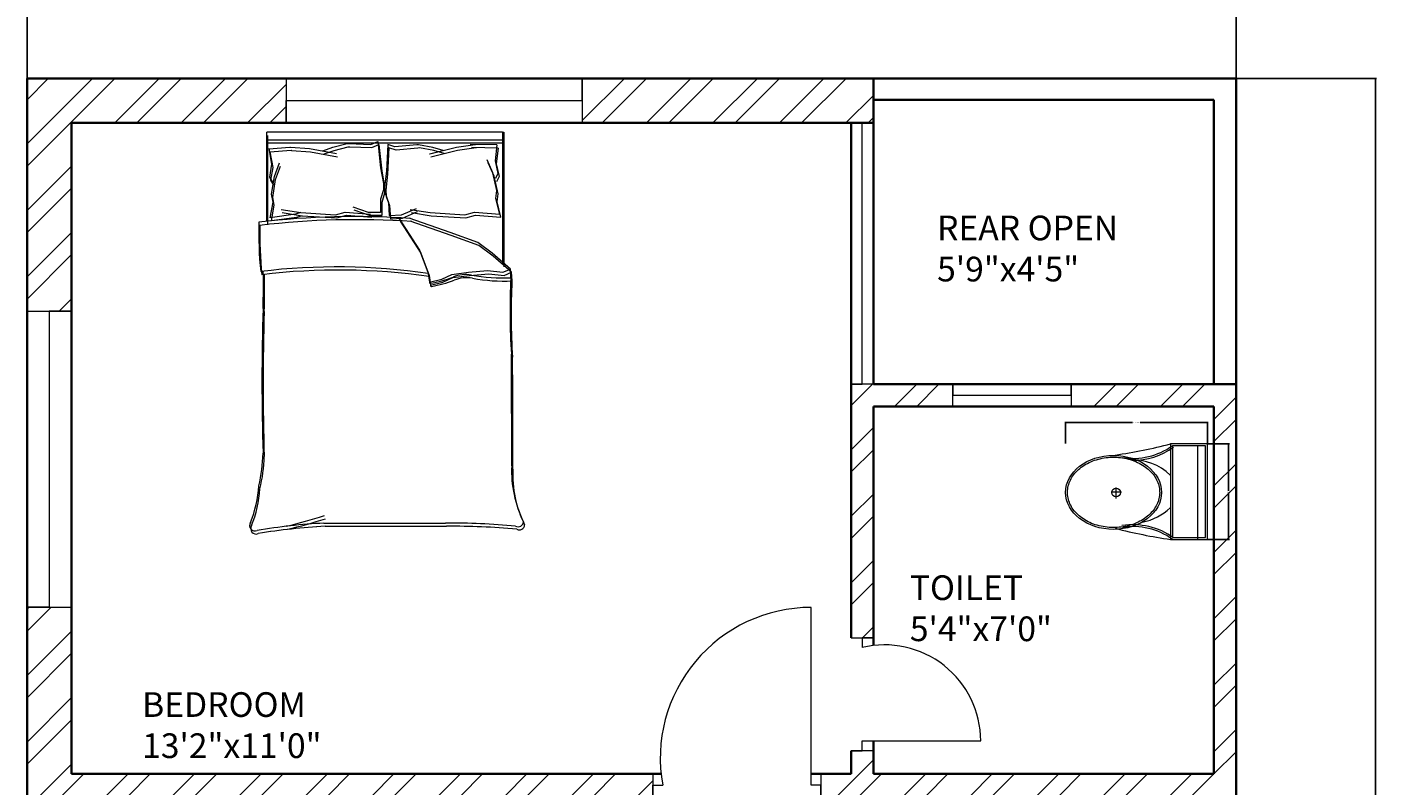
# Model space of a CAD drawing. Units: inches. Extents: x 1850 to 3445, y 1558 to 2756.
# Tile 7 of 13: x 2351 to 2625, y 2073 to 2227. Entities that reach past the tile are written whole.
import ezdxf

# ---------------------------------------------------------------- set-up
doc = ezdxf.new("R2010")
doc.units = ezdxf.units.IN
for name, color, linetype, lineweight in [('A-ANNO-DIMS', 2, 'Continuous', 18), ('A-AREA-IDEN', 7, 'Continuous', 18), ('A-DOOR', 3, 'Continuous', 18), ('A-FLOR-FIXT', 9, 'Continuous', 18), ('A-FURN', 8, 'Continuous', 13), ('A-GLAZ', 4, 'Continuous', 18), ('A-WALL', 7, 'Continuous', 35), ('A-WALL-PATT', 252, 'Continuous', 13)]:
    doc.layers.add(name, color=color, linetype=linetype, lineweight=lineweight)
doc.styles.get("Standard").update_dxf_attribs({"font": 'arial.ttf'})
doc.dimstyles.get("Standard").update_dxf_attribs({"dimtxt": 0.18, "dimasz": 0.18, "dimexe": 0.18, "dimexo": 0.0625, "dimgap": 0.09, "dimtad": 0, "dimtih": 1, "dimtoh": 1, "dimdec": 4, "dimzin": 0, "dimdsep": 46, "dimtxsty": 'Standard', "dimcen": 0.09, "dimadec": 0, "dimazin": 0, "dimtfac": 1, "dimtdec": 4, "dimtofl": 0, "dimtmove": 0, "dimatfit": 3, "dimfxl": 1, "dimtolj": 1, "dimtzin": 0, "dimarcsym": 0})

# ---------------------------------------------------------------- blocks, each defined once
blk = doc.blocks.new('A$C31115884')
for p, q in [((257.5, 466.4), (257.5, 523.2)), ((283.1, 497.7), (223.4, 497.7)), ((0, 200), (0, 0)), ((520, 200), (0, 200)), ((10, 190), (10, 10)), ((510, 190), (10, 190)), ((510, 10), (510, 190)), ((520, 0), (520, 200)), ((510, 54.5), (0, 54.5)), ((10, 10), (510, 10)), ((0, 0), (520, 0))]:
    blk.add_line(p, q)
blk.add_circle((255.6, 496.4), 23.6)
for centre, radius, start, end in [((2777.7, -204.6), 2807, 165.4549, 171.71327), ((-294.5, 403.3), 364.7, 324.20913, 9.34987), ((-294.5, 403.3), 374.7, 324.20913, 9.34987), ((805.8, 403.3), 364.7, 170.65013, 215.79087), ((3237, 905), 2807, 188.28673, 194.5451), ((139.5, 406.2), 293.5, 315.84364, 2.65635), ((805.8, 403.3), 374.7, 179.20365, 215.79087), ((383.6, 406.2), 293.5, 190.27735, 224.15636)]:
    blk.add_arc(centre, radius, start, end)
blk.add_ellipse((256.2, 509.9), major_axis=(0, -260.7), ratio=0.772727)
blk.add_open_spline([(256.2, 259.2), (263.1, 259.2), (270, 259.7), (287.8, 262.3), (298.7, 265.1), (319.9, 273.1), (330.2, 278.4), (350.1, 291.1), (359.7, 298.7), (377.7, 315.9), (386.2, 325.5), (401.7, 346.6), (408.8, 358.1), (421.3, 382.5), (426.8, 395.5), (435.9, 422.4), (439.5, 436.4), (444.8, 465.1), (446.5, 479.7), (447.9, 509.2), (447.6, 524), (445, 553.3), (442.7, 567.8), (436.3, 596), (432.1, 609.7), (421.9, 636), (416, 648.6), (402.5, 672.1), (395, 683), (378.6, 703), (369.8, 712.1), (351.1, 728), (341.3, 734.8), (320.9, 746.2), (310.4, 750.7), (288.9, 757.3), (278, 759.4), (256, 761), (245, 760.6), (223.1, 757.2), (212.3, 754.3), (191.1, 746.1), (180.8, 740.7), (160.9, 727.8), (151.4, 720.1), (133.5, 702.7), (125.1, 693), (109.6, 671.7), (102.6, 660.2), (90.2, 635.7), (84.9, 622.7), (76, 595.6), (72.4, 581.6), (67.2, 552.9), (65.6, 538.2), (64.4, 508.8), (64.8, 494), (67.5, 464.7), (69.9, 450.2), (76.6, 422), (80.8, 408.3), (91.1, 382.2), (97.2, 369.7), (110.8, 346.3), (118.4, 335.4), (134.8, 315.6), (143.7, 306.7), (162.4, 290.9), (172.3, 284.2), (192.8, 273), (203.3, 268.6), (224.8, 262.2), (235.8, 260.2), (249.9, 259.3), (253, 259.2), (256.2, 259.2)], degree=3, knots=[0, 0, 0, 0, 0.110105, 0.110105, 0.285049, 0.285049, 0.459994, 0.459994, 0.634938, 0.634938, 0.809882, 0.809882, 0.984827, 0.984827, 1.159771, 1.159771, 1.334715, 1.334715, 1.50966, 1.50966, 1.684604, 1.684604, 1.859549, 1.859549, 2.034493, 2.034493, 2.209437, 2.209437, 2.384382, 2.384382, 2.559326, 2.559326, 2.73427, 2.73427, 2.909215, 2.909215, 3.084159, 3.084159, 3.259103, 3.259103, 3.434048, 3.434048, 3.608992, 3.608992, 3.783936, 3.783936, 3.958881, 3.958881, 4.133825, 4.133825, 4.30877, 4.30877, 4.483714, 4.483714, 4.658658, 4.658658, 4.833603, 4.833603, 5.008547, 5.008547, 5.183491, 5.183491, 5.358436, 5.358436, 5.53338, 5.53338, 5.708324, 5.708324, 5.883269, 5.883269, 6.058213, 6.058213, 6.233158, 6.233158, 6.283185, 6.283185, 6.283185, 6.283185])
blk = doc.blocks.new('BED-PLAN')
for p, q in [((3.47, 63.33), (3.47, 81.44)), ((3.47, 79.91), (51.27, 79.91)), ((3.48, 63.33), (3.48, 81.44)), ((51.27, 81.44), (3.48, 81.44)), ((3.48, 79.91), (51.27, 79.91)), ((3.7, 62.69), (3.7, 80.8)), ((3.7, 62.69), (3.7, 80.8)), ((24.54, 78.99), (25.98, 79.57)), ((24.54, 78.99), (25.98, 79.57)), ((25.98, 79.57), (26.56, 74.22)), ((25.98, 79.57), (26.56, 74.22)), ((51.27, 81.44), (51.27, 54.83)), ((51.27, 81.44), (51.27, 54.83)), ((51.27, 81.44), (51.49, 81.44)), ((51.49, 81.44), (51.49, 80.8)), ((51.49, 80.8), (51.49, 54.19)), ((51.49, 80.8), (51.49, 54.19)), ((3.7, 79.27), (51.49, 79.27)), ((3.7, 79.27), (51.49, 79.27)), ((3.89, 78.13), (4.47, 74.95)), ((3.89, 78.13), (4.47, 74.95)), ((3.9, 78.11), (8.18, 78.43)), ((3.9, 78.11), (8.18, 78.43)), ((4.12, 77.49), (4.7, 74.31)), ((4.12, 77.49), (4.7, 74.31)), ((4.13, 77.47), (8.41, 77.8)), ((4.13, 77.47), (8.41, 77.8)), ((8.18, 78.43), (8.28, 78.42)), ((8.18, 78.43), (8.28, 78.42)), ((8.28, 78.42), (12.11, 78.13)), ((8.28, 78.42), (12.11, 78.13)), ((8.41, 77.8), (8.51, 77.78)), ((8.41, 77.8), (8.51, 77.78)), ((8.51, 77.78), (12.34, 77.49)), ((8.51, 77.78), (12.34, 77.49)), ((12.11, 78.13), (17.6, 77.11)), ((12.11, 78.13), (17.6, 77.11)), ((12.34, 77.49), (17.83, 76.48)), ((12.34, 77.49), (17.83, 76.48)), ((14.85, 77.69), (16.88, 78.42)), ((14.86, 77.69), (16.88, 78.42)), ((15.08, 77.05), (17.11, 77.78)), ((15.08, 77.05), (17.11, 77.78)), ((16.88, 78.42), (19.77, 79.14)), ((16.88, 78.42), (19.77, 79.14)), ((17.11, 77.78), (20, 78.5)), ((17.11, 77.78), (20, 78.5)), ((19.77, 79.14), (20.09, 79.14)), ((19.77, 79.14), (20.09, 79.14)), ((20, 78.5), (20.32, 78.5)), ((20, 78.5), (20.32, 78.5)), ((20.09, 79.14), (24.54, 78.99)), ((20.09, 79.14), (24.54, 78.99)), ((20.32, 78.5), (24.77, 78.36)), ((20.32, 78.5), (24.77, 78.36)), ((24.77, 78.36), (26.21, 78.93)), ((24.77, 78.36), (26.21, 78.93)), ((26.21, 78.93), (26.79, 73.58)), ((26.21, 78.93), (26.79, 73.58)), ((27.98, 78.95), (27.73, 73.58)), ((27.98, 78.95), (27.73, 73.58)), ((28.21, 78.31), (27.96, 72.94)), ((28.21, 78.31), (27.96, 72.94)), ((29.46, 78.46), (27.98, 78.95)), ((29.46, 78.46), (27.98, 78.95)), ((29.68, 77.83), (28.21, 78.31)), ((29.68, 77.83), (28.21, 78.31)), ((33.88, 78.89), (29.46, 78.46)), ((33.88, 78.89), (29.46, 78.46)), ((34.11, 78.25), (29.68, 77.83)), ((34.11, 78.25), (29.68, 77.83)), ((34.2, 78.91), (33.88, 78.89)), ((34.2, 78.91), (33.88, 78.89)), ((34.43, 78.27), (34.11, 78.25)), ((34.43, 78.27), (34.11, 78.25)), ((37.14, 78.36), (34.2, 78.91)), ((37.14, 78.36), (34.2, 78.91)), ((37.36, 77.73), (34.43, 78.27)), ((37.36, 77.73), (34.43, 78.27)), ((41.91, 78.37), (36.49, 77.02)), ((41.91, 78.37), (36.5, 77.02)), ((42.14, 77.73), (36.72, 76.38)), ((42.14, 77.73), (36.72, 76.38)), ((39.2, 77.77), (37.14, 78.36)), ((39.2, 77.77), (37.14, 78.36)), ((39.43, 77.13), (37.36, 77.73)), ((39.43, 77.13), (37.36, 77.73)), ((45.71, 78.9), (41.91, 78.37)), ((45.71, 78.9), (41.91, 78.37)), ((45.94, 78.26), (42.14, 77.73)), ((45.94, 78.26), (42.14, 77.73)), ((50.11, 78.89), (44.71, 78.98)), ((44.71, 78.98), (45.71, 78.9)), ((50.11, 78.89), (44.71, 78.98)), ((44.71, 78.98), (45.71, 78.9)), ((50.34, 78.25), (44.94, 78.34)), ((44.94, 78.34), (45.94, 78.26)), ((50.34, 78.25), (44.94, 78.34)), ((44.94, 78.34), (45.94, 78.26)), ((50.11, 78.89), (49.73, 75.68)), ((50.11, 78.89), (49.73, 75.68)), ((50.34, 78.25), (49.96, 75.04)), ((50.34, 78.25), (49.96, 75.04)), ((4.47, 74.95), (4.04, 72.34)), ((4.47, 74.95), (4.04, 72.34)), ((4.7, 74.31), (4.27, 71.7)), ((4.7, 74.31), (4.27, 71.7)), ((5.05, 72.49), (6.06, 75.24)), ((5.05, 72.49), (6.06, 75.24)), ((5.28, 71.85), (6.29, 74.6)), ((5.28, 71.85), (6.29, 74.6)), ((26.56, 74.22), (27.14, 71.04)), ((26.56, 74.22), (27.14, 71.04)), ((49.31, 73.19), (48.13, 75.86)), ((49.31, 73.19), (48.13, 75.86)), ((49.54, 72.55), (48.36, 75.23)), ((49.54, 72.55), (48.36, 75.23)), ((49.73, 75.68), (50.33, 73.1)), ((49.73, 75.68), (50.33, 73.1)), ((49.96, 75.04), (50.56, 72.47)), ((49.96, 75.04), (50.56, 72.47)), ((4.04, 72.34), (4.62, 71.33)), ((4.04, 72.34), (4.62, 71.33)), ((4.27, 71.7), (4.85, 70.69)), ((4.27, 71.7), (4.85, 70.69)), ((4.47, 68.87), (5.05, 72.49)), ((4.47, 68.87), (5.05, 72.49)), ((4.7, 68.23), (5.28, 71.85)), ((4.7, 68.23), (5.28, 71.85)), ((26.79, 73.58), (27.37, 70.4)), ((26.79, 73.58), (27.37, 70.4)), ((27.73, 73.58), (27.35, 70.37)), ((27.73, 73.58), (27.35, 70.37)), ((27.96, 72.94), (27.58, 69.73)), ((27.96, 72.94), (27.58, 69.73)), ((50.11, 69.61), (49.31, 73.19)), ((50.11, 69.61), (49.31, 73.19)), ((50.34, 68.98), (49.54, 72.55)), ((50.34, 68.98), (49.54, 72.55)), ((50.33, 73.1), (49.81, 72.06)), ((50.33, 73.1), (49.81, 72.06)), ((50.56, 72.47), (50.04, 71.42)), ((50.56, 72.47), (50.04, 71.42)), ((4.76, 67.28), (4.47, 68.87)), ((4.76, 67.28), (4.47, 68.87)), ((27.14, 69.74), (26.56, 67.86)), ((27.14, 69.74), (26.56, 67.86)), ((27.37, 69.1), (26.79, 67.22)), ((27.37, 69.1), (26.79, 67.22)), ((27.14, 71.04), (27.14, 69.74)), ((27.14, 71.04), (27.14, 69.74)), ((27.35, 70.37), (27.44, 69.07)), ((27.35, 70.37), (27.44, 69.07)), ((27.37, 70.4), (27.37, 69.1)), ((27.37, 70.4), (27.37, 69.1)), ((27.44, 69.07), (28.13, 67.23)), ((27.44, 69.07), (28.13, 67.23)), ((27.58, 69.73), (27.66, 68.43)), ((27.58, 69.73), (27.66, 68.43)), ((27.66, 68.43), (28.36, 66.59)), ((27.66, 68.43), (28.36, 66.59)), ((49.92, 68.01), (50.11, 69.61)), ((49.92, 68.01), (50.11, 69.61)), ((50.15, 67.37), (50.34, 68.98)), ((50.15, 67.37), (50.34, 68.98)), ((4.18, 64.1), (4.76, 67.28)), ((4.18, 64.1), (4.76, 67.28)), ((4.41, 63.46), (4.99, 66.64)), ((4.41, 63.46), (4.99, 66.64)), ((4.99, 66.64), (4.7, 68.23)), ((4.99, 66.64), (4.7, 68.23)), ((6.38, 65.81), (10.41, 65.15)), ((6.38, 65.81), (10.41, 65.15)), ((24.1, 65.18), (20.96, 66.27)), ((24.1, 65.18), (20.96, 66.27)), ((26.56, 67.86), (26.56, 65.18)), ((26.56, 67.86), (26.56, 65.18)), ((26.79, 67.22), (26.79, 64.54)), ((26.79, 67.22), (26.79, 64.54)), ((28.13, 67.23), (28.3, 64.55)), ((28.13, 67.23), (28.3, 64.55)), ((28.36, 66.59), (28.53, 63.91)), ((28.36, 66.59), (28.53, 63.91)), ((30.75, 64.7), (33.82, 65.99)), ((30.75, 64.7), (33.82, 65.99)), ((32.56, 65.81), (36.6, 65.15)), ((32.56, 65.81), (36.6, 65.15)), ((50.7, 64.87), (49.92, 68.01)), ((50.7, 64.87), (49.92, 68.01)), ((50.93, 64.23), (50.15, 67.37)), ((50.93, 64.23), (50.15, 67.37)), ((9.28, 64.83), (4.18, 64.1)), ((9.28, 64.83), (4.18, 64.1)), ((9.51, 64.19), (4.41, 63.46)), ((9.51, 64.19), (4.41, 63.46)), ((6.61, 65.18), (10.64, 64.51)), ((6.61, 65.18), (10.64, 64.51)), ((10.41, 65.15), (9.28, 64.83)), ((10.41, 65.15), (9.28, 64.83)), ((10.64, 64.51), (9.51, 64.19)), ((10.64, 64.51), (9.51, 64.19)), ((10.41, 65.15), (17.42, 64.72)), ((10.41, 65.15), (17.42, 64.72)), ((10.64, 64.51), (17.65, 64.08)), ((10.64, 64.51), (17.65, 64.08)), ((17.42, 64.72), (19.38, 65.27)), ((17.42, 64.72), (19.38, 65.27)), ((17.65, 64.08), (19.61, 64.63)), ((17.65, 64.08), (19.61, 64.63)), ((19.38, 65.27), (24.52, 64.87)), ((19.38, 65.27), (24.52, 64.87)), ((19.61, 64.63), (24.74, 64.23)), ((19.61, 64.63), (24.74, 64.23)), ((24.33, 64.54), (21.19, 65.63)), ((24.33, 64.54), (21.19, 65.63)), ((26.56, 65.18), (24.1, 65.18)), ((26.56, 65.18), (24.1, 65.18)), ((26.79, 64.54), (24.33, 64.54)), ((26.79, 64.54), (24.33, 64.54)), ((28.3, 64.55), (30.75, 64.7)), ((28.3, 64.55), (30.75, 64.7)), ((28.53, 63.91), (30.98, 64.06)), ((28.53, 63.91), (30.98, 64.06)), ((30.26, 64.06), (34.45, 57.57)), ((30.26, 64.06), (34.45, 57.57)), ((30.49, 63.42), (34.68, 56.93)), ((30.49, 63.42), (34.68, 56.93)), ((30.98, 64.06), (34.05, 65.35)), ((30.98, 64.06), (34.05, 65.35)), ((40.64, 61.13), (32.31, 64.06)), ((40.64, 61.13), (32.31, 64.06)), ((40.87, 60.49), (32.53, 63.42)), ((40.87, 60.49), (32.53, 63.42)), ((32.79, 65.18), (36.82, 64.51)), ((32.79, 65.18), (36.82, 64.51)), ((36.6, 65.15), (43.61, 64.72)), ((36.6, 65.15), (43.61, 64.72)), ((36.82, 64.51), (43.83, 64.08)), ((36.82, 64.51), (43.83, 64.08)), ((43.61, 64.72), (45.57, 65.27)), ((43.61, 64.72), (45.57, 65.27)), ((43.83, 64.08), (45.79, 64.63)), ((43.83, 64.08), (45.79, 64.63)), ((45.57, 65.27), (50.7, 64.87)), ((45.57, 65.27), (50.7, 64.87)), ((45.79, 64.63), (50.93, 64.23)), ((45.79, 64.63), (50.93, 64.23)), ((46.22, 59.11), (40.64, 61.13)), ((46.22, 59.11), (40.64, 61.13)), ((46.45, 58.48), (40.87, 60.49)), ((46.45, 58.48), (40.87, 60.49)), ((34.45, 57.57), (36.15, 53.08)), ((34.45, 57.57), (36.15, 53.08)), ((49.16, 56.95), (46.22, 59.11)), ((49.16, 56.95), (46.22, 59.11)), ((49.39, 56.31), (46.45, 58.48)), ((49.39, 56.31), (46.45, 58.48)), ((34.68, 56.93), (36.38, 52.44)), ((34.68, 56.93), (36.38, 52.44)), ((52.87, 53.7), (49.16, 56.95)), ((52.87, 53.7), (49.16, 56.95)), ((53.1, 53.06), (49.39, 56.31)), ((53.1, 53.06), (49.39, 56.31)), ((36.15, 53.08), (36.46, 51.07)), ((36.15, 53.08), (36.46, 51.07)), ((36.38, 52.44), (36.69, 50.43)), ((36.38, 52.44), (36.69, 50.43)), ((38.94, 51.69), (40.95, 52.61)), ((38.94, 51.69), (40.95, 52.61)), ((40.95, 52.61), (44.36, 53.08)), ((40.95, 52.61), (44.36, 53.08)), ((41.18, 51.97), (44.59, 52.44)), ((41.18, 51.97), (44.59, 52.44)), ((44.36, 53.08), (48.23, 53.39)), ((44.36, 53.08), (48.23, 53.39)), ((44.59, 52.44), (48.46, 52.75)), ((44.59, 52.44), (48.46, 52.75)), ((48.23, 53.39), (51.33, 53.08)), ((48.23, 53.39), (51.33, 53.08)), ((48.46, 52.75), (51.56, 52.44)), ((48.46, 52.75), (51.56, 52.44)), ((51.33, 53.08), (52.87, 53.7)), ((51.33, 53.08), (52.87, 53.7)), ((51.56, 52.44), (53.1, 53.06)), ((51.56, 52.44), (53.1, 53.06)), ((52.95, 51.95), (52.87, 53.7, 3.87)), ((52.95, 51.95), (52.87, 53.7, 3.87)), ((53.18, 51.31), (53.1, 53.06, 3.87)), ((53.18, 51.31), (53.1, 53.06, 3.87)), ((36.46, 51.07), (38.94, 51.69)), ((36.46, 51.07), (38.94, 51.69)), ((36.69, 50.43), (39.17, 51.05)), ((36.69, 50.43), (39.17, 51.05)), ((39.17, 51.05), (41.18, 51.97)), ((39.17, 51.05), (41.18, 51.97)), ((15.06, 2.2), (39.68, 2.2)), ((15.06, 2.2), (39.68, 2.2)), ((15.29, 1.56), (39.91, 1.56)), ((15.29, 1.56), (39.91, 1.56))]:
    blk.add_line(p, q)
for centre, radius, start, end in [((85.16, 61.35), 83.31, 178.7218, 185.604), ((85.16, 61.35), 83.31, 178.7218, 185.604), ((21.36, -100.61), 164.97, 86.0865, 96.7821), ((21.36, -100.61), 164.97, 86.0865, 96.7821), ((21.59, -101.25), 164.97, 86.0865, 96.7821), ((21.59, -101.25), 164.97, 86.0865, 96.7821), ((85.39, 60.71), 83.31, 178.7218, 185.604), ((85.39, 60.71), 83.31, 178.7218, 185.604), ((17.76, -74.87), 129.02, 81.7845, 96.9006), ((17.76, -74.87), 129.02, 81.7845, 96.9006), ((17.98, -75.51), 129.02, 81.7845, 96.9006), ((17.98, -75.51), 129.02, 81.7845, 96.9006), ((-167.31, 50.27), 170.11, 358.4762, 1.0082), ((-167.31, 50.27), 170.11, 358.4762, 1.0082), ((-167.08, 49.63), 170.11, 358.4762, 1.0082), ((-167.08, 49.63), 170.11, 358.4762, 1.0082), ((31.15, 79.96), 29.65, 280.6617, 289.8806), ((31.15, 79.96), 29.65, 280.6617, 289.8806), ((43.74, 46.38), 6.22, 78.6608, 113.7384), ((43.74, 46.38), 6.22, 78.6608, 113.7384), ((51.33, 88.1), 36.18, 259.8763, 272.5657), ((51.33, 88.1), 36.18, 259.8763, 272.5657), ((36.64, 51), 0.185, 160.2464, 271.1377), ((36.64, 51), 0.185, 160.2464, 271.1377), ((36.86, 50.36), 0.185, 160.2464, 271.1377), ((36.86, 50.36), 0.185, 160.2464, 271.1377), ((31.38, 79.32), 29.65, 280.6617, 289.8806), ((31.38, 79.32), 29.65, 280.6617, 289.8806), ((43.97, 45.74), 6.22, 78.6608, 113.7384), ((43.97, 45.74), 6.22, 78.6608, 113.7384), ((51.56, 87.46), 36.18, 259.8763, 272.5657), ((51.56, 87.46), 36.18, 259.8763, 272.5657), ((182.27, 45.13), 129.5, 176.9791, 183.8365), ((182.27, 45.13), 129.5, 176.9791, 183.8365), ((182.49, 44.49), 129.5, 176.9791, 183.8365), ((182.49, 44.49), 129.5, 176.9791, 183.8365), ((484.82, 30.83), 482.31, 178.2277, 181.7185), ((484.82, 30.83), 482.31, 178.2277, 181.7185), ((485.05, 30.19), 482.31, 178.2277, 181.7185), ((485.05, 30.19), 482.31, 178.2277, 181.7185), ((-4508.74, 13.62), 4561.86, 0.00217, 0.28689), ((-4508.74, 13.62), 4561.86, 0.00217, 0.28689), ((-4508.51, 12.98), 4561.86, 0.00217, 0.28689), ((-4508.52, 12.98), 4561.86, 0.00217, 0.28689), ((-26.9, 16.93), 29.63, 346.0648, 358.9113), ((-26.9, 16.93), 29.63, 346.0648, 358.9113), ((-26.67, 16.29), 29.63, 346.0648, 358.9113), ((-26.67, 16.29), 29.63, 346.0648, 358.9113), ((76.16, 12.78), 23.07, 177.4714, 206.4681), ((76.16, 12.78), 23.07, 177.4714, 206.4681), ((76.39, 12.14), 23.07, 177.4714, 206.4681), ((76.39, 12.14), 23.07, 177.4714, 206.4681), ((-21.66, 11.17), 23.56, 337.9751, 356.652), ((-21.66, 11.17), 23.56, 337.9751, 356.652), ((-21.43, 10.53), 23.56, 337.9751, 356.652), ((-21.43, 10.53), 23.56, 337.9751, 356.652), ((-17.22, 105.16), 106.46, 283.3832, 287.7053), ((-17.22, 105.16), 106.46, 283.3832, 287.7053), ((-16.99, 104.52), 106.46, 283.3832, 287.7053), ((-16.99, 104.52), 106.46, 283.3832, 287.7053), ((1.09, 1.73), 1.09, 146.1736, 293.4781), ((1.09, 1.73), 1.09, 146.1736, 293.4781), ((1.32, 1.09), 1.09, 146.1736, 293.4781), ((1.32, 1.09), 1.09, 146.1736, 293.4781), ((21.43, -119.39), 121.76, 92.9958, 99.4091), ((21.43, -119.39), 121.76, 92.9958, 99.4091), ((21.66, -120.03), 121.76, 92.9958, 99.4091), ((21.65, -120.03), 121.76, 92.9958, 99.4091), ((41.15, -130.83), 133.04, 84.4998, 90.6351), ((41.15, -130.83), 133.04, 84.4998, 90.6351), ((41.38, -131.47), 133.04, 84.4998, 90.6351), ((41.38, -131.47), 133.04, 84.4998, 90.6351), ((54.41, 2.57), 1.1, 242.6588, 356.02), ((54.41, 2.57), 1.1, 242.6588, 356.02), ((54.64, 1.93), 1.1, 242.6588, 356.02), ((54.64, 1.93), 1.1, 242.6588, 356.02)]:
    blk.add_arc(centre, radius, start, end)
blk = doc.blocks.new('WIN-60-W9')
for p, q in [((0, 9), (0, 0)), ((60, 4.5), (60, 9)), ((60, 9), (60, 0)), ((0, 0), (0, 4.5)), ((0, 4.5), (60, 4.5))]:
    blk.add_line(p, q)
blk = doc.blocks.new('WIN-24-W4_5')
for p, q in [((0, 0), (0, 4.5)), ((0, 4.5), (0, 2.25)), ((24, 2.25), (24, 4.5)), ((24, 4.5), (24, 0)), ((0, 2.25), (24, 2.25))]:
    blk.add_line(p, q)
blk = doc.blocks.new('DOOR-BATH-REAR-UPPER')
for p, q in [((0, 22.93), (4.5, 22.93)), ((4.5, 22.93), (2.25, 22.93)), ((2.25, 22.93), (2.25, 20.93)), ((2.25, 0), (2.25, 2)), ((2.25, 2), (26.25, 2)), ((4.5, 0), (0, 0)), ((0, 0), (2.25, 0))]:
    blk.add_line(p, q)
blk.add_arc((6.78, 2), 19.47, 0, 103.4712)
blk = doc.blocks.new('DOOR-BED-UPPER')
for p, q in [((32.07, 2.25), (32.07, 38.25)), ((0, 4.5), (0, 0)), ((34.07, 4.5), (34.07, 0)), ((0, 0), (0, 2.25)), ((0, 2.25), (2, 2.25)), ((34.07, 2.25), (32.07, 2.25)), ((34.07, 0), (34.07, 2.25))]:
    blk.add_line(p, q)
blk.add_arc((32.07, 7.69), 30.56, 90, 190.2532)
blk = doc.blocks.new('*D48')
at = {"layer": 'A-ANNO-DIMS', "color": 0, "lineweight": -2, "transparency": 16777216}
for p, q in [((2561.52, 2142.15), (2561.52, 2146.58)), ((2561.7, 2146.4), (2575.1, 2146.4)), ((2590.06, 2146.4), (2576.65, 2146.4)), ((2590.24, 2142.15), (2590.24, 2146.58))]:
    blk.add_line(p, q, dxfattribs=at)
at = {"layer": 'A-ANNO-DIMS', "color": 0, "transparency": 16777216}
for points in [[(2561.7, 2146.43), (2561.7, 2146.37), (2561.52, 2146.4)], [(2590.06, 2146.43), (2590.06, 2146.37), (2590.24, 2146.4)]]:
    blk.add_solid(points, dxfattribs=at)
at = {"layer": 'Defpoints', "color": 0, "transparency": 16777216}
for p in [(2561.52, 2146.4), (2561.52, 2142.09), (2590.24, 2142.09)]:
    blk.add_point(p, dxfattribs=at)
at = {"layer": 'A-ANNO-DIMS', "color": 0, "transparency": 16777216, "insert": (2575.88, 2146.4), "char_height": 0.18, "attachment_point": 5}
blk.add_mtext('\\A1;WC 29 TYP.', dxfattribs=at)
blk = doc.blocks.new('*D49')
at = {"layer": 'A-ANNO-DIMS', "color": 0, "lineweight": -2, "transparency": 16777216}
for p, q in [((2590.3, 2142.09), (2594.73, 2142.09)), ((2594.55, 2141.91), (2594.55, 2132.58)), ((2594.55, 2122.89), (2594.55, 2132.22)), ((2590.3, 2122.71), (2594.73, 2122.71))]:
    blk.add_line(p, q, dxfattribs=at)
at = {"layer": 'A-ANNO-DIMS', "color": 0, "transparency": 16777216}
for points in [[(2594.52, 2141.91), (2594.58, 2141.91), (2594.55, 2142.09)], [(2594.52, 2122.89), (2594.58, 2122.89), (2594.55, 2122.71)]]:
    blk.add_solid(points, dxfattribs=at)
at = {"layer": 'Defpoints', "color": 0, "transparency": 16777216}
for p in [(2590.24, 2142.09), (2594.55, 2142.09), (2590.24, 2122.71)]:
    blk.add_point(p, dxfattribs=at)
at = {"layer": 'A-ANNO-DIMS', "color": 0, "transparency": 16777216, "insert": (2594.55, 2132.4), "char_height": 0.18, "attachment_point": 5}
blk.add_mtext('\\A1;19 TYP.', dxfattribs=at)
blk = doc.blocks.new('*D82')
at = {"layer": 'A-ANNO-DIMS', "color": 0, "lineweight": -2, "transparency": 16777216}
for p, q in [((2351.06, 2216.25), (2351.06, 2244.61)), ((2351.24, 2244.43), (2473.26, 2244.43)), ((2595.88, 2244.43), (2473.85, 2244.43)), ((2596.06, 2216.25), (2596.06, 2244.61))]:
    blk.add_line(p, q, dxfattribs=at)
at = {"layer": 'A-ANNO-DIMS', "color": 0, "transparency": 16777216}
for points in [[(2351.24, 2244.46), (2351.24, 2244.4), (2351.06, 2244.43)], [(2595.88, 2244.46), (2595.88, 2244.4), (2596.06, 2244.43)]]:
    blk.add_solid(points, dxfattribs=at)
at = {"layer": 'Defpoints', "color": 0, "transparency": 16777216}
for p in [(2596.06, 2244.43), (2351.06, 2216.18), (2596.06, 2216.18)]:
    blk.add_point(p, dxfattribs=at)
at = {"layer": 'A-ANNO-DIMS', "color": 0, "transparency": 16777216, "insert": (2473.56, 2244.43), "char_height": 0.18, "attachment_point": 5}
blk.add_mtext('\\A1;245', dxfattribs=at)
blk = doc.blocks.new('*D83')
at = {"layer": 'A-ANNO-DIMS', "color": 0, "lineweight": -2, "transparency": 16777216}
for p, q in [((2596.12, 2216.18), (2624.49, 2216.18)), ((2624.31, 2216), (2624.31, 1977.12)), ((2624.31, 1737.86), (2624.31, 1976.75)), ((2596.12, 1737.68), (2624.49, 1737.68))]:
    blk.add_line(p, q, dxfattribs=at)
at = {"layer": 'A-ANNO-DIMS', "color": 0, "transparency": 16777216}
for points in [[(2624.28, 2216), (2624.34, 2216), (2624.31, 2216.18)], [(2624.28, 1737.86), (2624.34, 1737.86), (2624.31, 1737.68)]]:
    blk.add_solid(points, dxfattribs=at)
at = {"layer": 'Defpoints', "color": 0, "transparency": 16777216}
for p in [(2596.06, 2216.18), (2624.31, 2216.18), (2596.06, 1737.68)]:
    blk.add_point(p, dxfattribs=at)
at = {"layer": 'A-ANNO-DIMS', "color": 0, "transparency": 16777216, "insert": (2624.31, 1976.93), "char_height": 0.18, "attachment_point": 5}
blk.add_mtext('\\A1;478.5', dxfattribs=at)

msp = doc.modelspace()

# ---------------------------------------------------------------- hatches: boundary and pattern name
at = {"layer": 'A-WALL-PATT'}
h = msp.add_hatch(dxfattribs=at)
h.set_pattern_fill('ANSI32', color=256)
h.paths.add_polyline_path([(2403.5576, 2211.6843), (2403.5576, 2216.1843), (2351.0556, 2216.1843), (2351.0556, 2169.0079), (2360.0556, 2169.0079), (2360.0556, 2207.1843), (2403.5576, 2207.1843)])
h.paths.add_polyline_path([(2522.5556, 2216.1843), (2463.5576, 2216.1843), (2463.5576, 2207.1843), (2522.5556, 2207.1843)])
h.paths.add_polyline_path([(2596.0556, 2154.1843), (2562.6647, 2154.1843), (2562.6647, 2149.6843), (2591.5556, 2149.6843), (2591.5556, 2075.1843), (2522.5556, 2075.1843), (2522.5556, 2079.8699), (2518.0556, 2079.8699), (2518.0556, 2075.1843), (2511.9412, 2075.1843), (2511.9412, 2070.6843), (2591.5556, 2070.6843), (2591.5556, 2036.4962), (2596.0556, 2036.4962)])
h.paths.add_polyline_path([(2538.6647, 2154.1843), (2522.5556, 2154.1843), (2518.0556, 2154.1843), (2518.0556, 2102.7998), (2522.5556, 2102.7998), (2522.5556, 2149.6843), (2538.6647, 2149.6843)], flags=17)
h.paths.add_polyline_path([(2477.8689, 2072.9343), (2477.8689, 2075.1843), (2360.0556, 2075.1843), (2360.0556, 2109.0079), (2355.5556, 2109.0079), (2351.0556, 2109.0079), (2351.0556, 2043.8694), (2355.5556, 2043.8694), (2360.0556, 2043.8694), (2360.0556, 2070.6843), (2450.0556, 2070.6843), (2450.0556, 2045.0271), (2454.5556, 2045.0271), (2454.5556, 2070.6843), (2477.8689, 2070.6843)])
h.paths.add_polyline_path([(2360.0556, 2007.8694), (2351.0556, 2007.8694), (2351.0556, 1958.9131), (2355.5556, 1958.9131), (2360.0556, 1958.9131), (2360.0556, 1970.1843), (2450.0556, 1970.1843), (2450.0556, 1913.1843), (2443.7332, 1913.1843), (2443.7332, 1908.6843), (2454.5556, 1908.6843), (2454.5556, 1999.4184), (2450.0556, 1999.4184), (2450.0556, 1974.6843), (2360.0556, 1974.6843)])
h.paths.add_polyline_path([(2360.0556, 1908.6843), (2422.4247, 1908.6843), (2422.4247, 1910.9343), (2422.4247, 1913.1843), (2360.0556, 1913.1843), (2360.0556, 1934.9131), (2351.0556, 1934.9131), (2351.0556, 1778.1843), (2426.033, 1778.1843), (2426.033, 1780.4343), (2426.033, 1782.6843), (2360.0556, 1782.6843)])
h.paths.add_polyline_path([(2515.0556, 1782.6843), (2486.033, 1782.6843), (2486.033, 1778.1843), (2515.0556, 1778.1843)])

# ---------------------------------------------------------------- linework, layer by layer
at = {"layer": 'A-GLAZ'}
for p, q in [((2520.3056, 2154.1843), (2520.3056, 2207.1843)), ((2522.5556, 2154.1843), (2518.0556, 2154.1843)), ((2518.0556, 2154.1843), (2520.3056, 2154.1843))]:
    msp.add_line(p, q, dxfattribs=at)
at = {"layer": 'A-WALL'}
for p, q in [((2351.0556, 2216.1843), (2596.0556, 2216.1843)), ((2351.0556, 2216.1843), (2351.0556, 1737.6843)), ((2522.5556, 2216.1843), (2522.5556, 2154.1843)), ((2596.0556, 2216.1843), (2596.0556, 1737.6843)), ((2522.5556, 2211.8264), (2591.5556, 2211.8264)), ((2591.5556, 2211.8264), (2591.5556, 2207.1843)), ((2360.0556, 2207.1843), (2522.5556, 2207.1843)), ((2360.0556, 2207.1843), (2360.0556, 2075.1843)), ((2518.0556, 2207.1843), (2518.0556, 2102.7998)), ((2591.5556, 2207.1843), (2591.5556, 2154.1843)), ((2522.5556, 2154.1843), (2596.0556, 2154.1843)), ((2522.5556, 2149.6843), (2522.5556, 2101.2008)), ((2522.5556, 2149.6843), (2591.5556, 2149.6843)), ((2591.5556, 2149.6843), (2591.5556, 2075.1843)), ((2522.5556, 2081.8699), (2522.5556, 2075.1843)), ((2518.0556, 2079.8699), (2518.0556, 2075.1843)), ((2360.0556, 2075.1843), (2479.5478, 2075.1843)), ((2509.9412, 2075.1843), (2518.0556, 2075.1843)), ((2522.5556, 2075.1843), (2591.5556, 2075.1843))]:
    msp.add_line(p, q, dxfattribs=at)

# ---------------------------------------------------------------- block references
at = {"layer": 'A-DOOR'}
for name, p in [('DOOR-BED-UPPER', (2477.869, 2070.684)), ('DOOR-BATH-REAR-UPPER', (2518.056, 2079.87))]:
    msp.add_blockref(name, p, dxfattribs=at)
at = {"layer": 'A-FLOR-FIXT', "xscale": 0.0372717239612423, "yscale": 0.0372717239612423, "zscale": 0.0372717239612423, "rotation": 89.99999999999999}
msp.add_blockref('A$C31115884', (2590.237, 2122.708), dxfattribs=at)
at = {"layer": 'A-FURN'}
msp.add_blockref('BED-PLAN', (2396.1595, 2123.8152), dxfattribs=at)
at = {"layer": 'A-GLAZ'}
for name, p in [('WIN-60-W9', (2403.5575, 2207.184)), ('WIN-24-W4_5', (2538.665, 2149.684))]:
    msp.add_blockref(name, p, dxfattribs=at)
at = {"layer": 'A-GLAZ', "extrusion": (0, 0, -1), "zscale": -1, "rotation": 270}
msp.add_blockref('WIN-60-W9', (-2360.0559, 2169.008), dxfattribs=at)

# ---------------------------------------------------------------- texts
at = {"layer": 'A-AREA-IDEN', "char_height": 5, "attachment_point": 1}
for s, width, insert in [('REAR OPEN\\P5\'9"x4\'5"', 101.614587, (2535.4723, 2188.358)), ('TOILET\\P5\'4"x7\'0"', 115.801334, (2529.9458, 2115.4354)), ('BEDROOM\\P13\'2"x11\'0"', 157.927169, (2374.3784, 2091.7435))]:
    msp.add_mtext_dynamic_manual_height_columns(s, width=width, gutter_width=12.5, heights=[0], dxfattribs=dict(at, insert=insert))

# ---------------------------------------------------------------- dimensions: what is measured, and where the dimension line sits
at = {"layer": 'A-ANNO-DIMS'}
dim = msp.add_linear_dim(base=(2596.0556, 2244.4343), p1=(2351.0556, 2216.1843), p2=(2596.0556, 2216.1843), dimstyle='Standard', override={"dimdec": 0, "dimlfac": 1, "dimrnd": 0, "dimzin": 0, "dimdsep": 46, "dimlunit": 2}, dxfattribs=at)
dim.commit()
dim.dimension.update_dxf_attribs({"geometry": '*D82', "text_midpoint": (2473.5556, 2244.4343)})
dim = msp.add_linear_dim(base=(2624.3056, 2216.1843), p1=(2596.0556, 1737.6843), p2=(2596.0556, 2216.1843), angle=90, dimstyle='Standard', override={"dimdec": 1, "dimlfac": 1, "dimrnd": 0, "dimzin": 0, "dimdsep": 46, "dimlunit": 2}, dxfattribs=at)
dim.commit()
dim.dimension.update_dxf_attribs({"geometry": '*D83', "text_midpoint": (2624.3056, 1976.9343)})
for base, p1, p2, angle, text, picture, middle in [((2561.5165, 2146.3974), (2590.237, 2142.0893), (2561.5165, 2142.0893), 180, 'WC <> TYP.', '*D48', (2575.8767, 2146.3974)), ((2594.545, 2142.0893), (2590.237, 2122.708), (2590.237, 2142.0893), 90, '<> TYP.', '*D49', (2594.545, 2132.3987))]:
    dim = msp.add_linear_dim(base=base, p1=p1, p2=p2, angle=angle, text=text, dimstyle='Standard', override={"dimdec": 0, "dimlfac": 1, "dimrnd": 0, "dimzin": 0, "dimdsep": 46, "dimlunit": 2}, dxfattribs=at)
    dim.commit()
    dim.dimension.update_dxf_attribs({"geometry": picture, "text_midpoint": middle})

doc.saveas('drawing.dxf')
